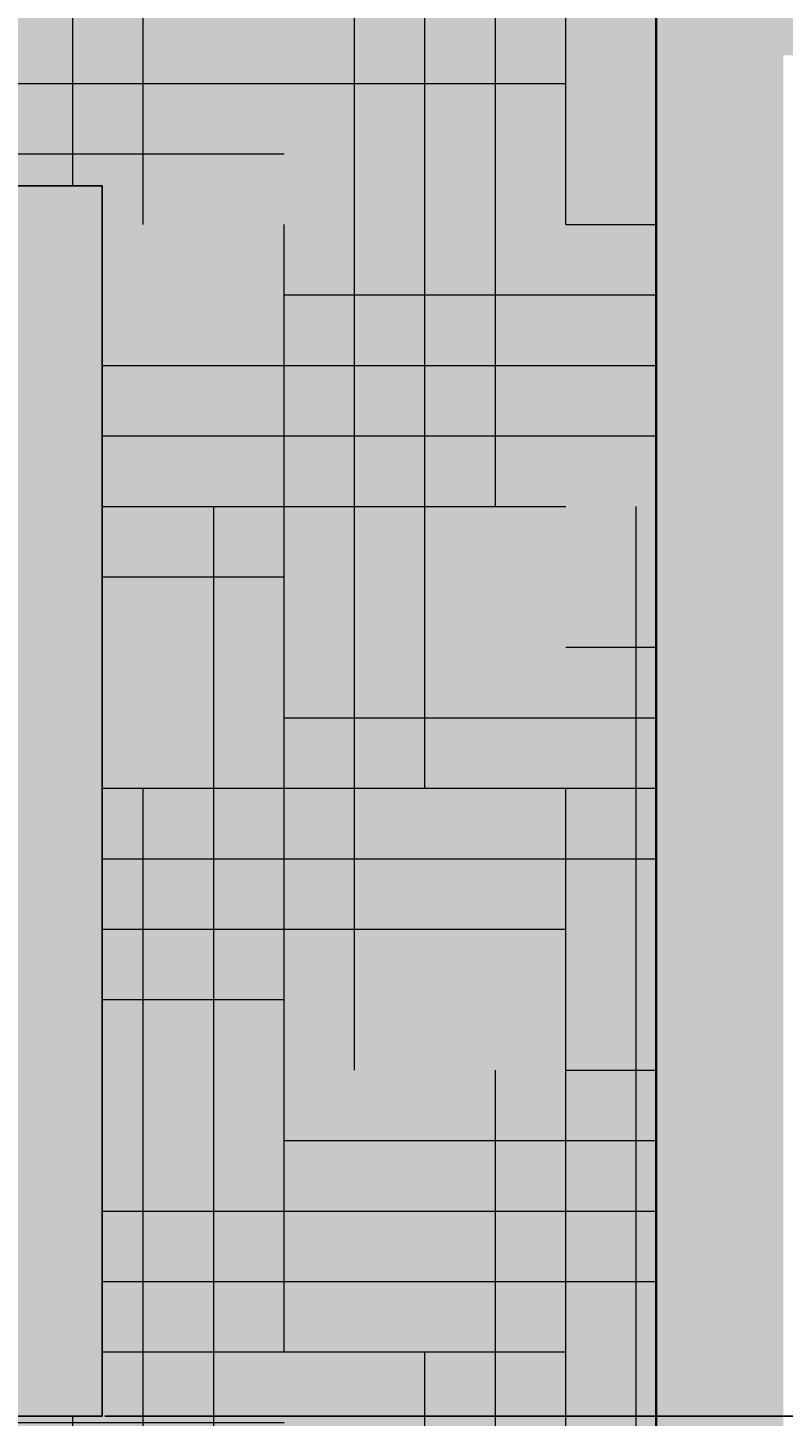
# Model space of a CAD drawing. Units: feet. Extents: x 2695 to 2912, y 795 to 1139.
# Tile 13 of 83: x 2756 to 2774, y 875 to 906. Entities that reach past the tile are written whole.
import ezdxf

# ---------------------------------------------------------------- set-up
doc = ezdxf.new("R2010")
doc.units = ezdxf.units.FT
for name, color, linetype, lineweight in [('A-ANNO-DIMS', 2, 'Continuous', 18), ('A-ELEV', 7, 'Continuous', 35), ('A-ELEV-PATT', 252, 'Continuous', 13), ('A-GLAZ', 4, 'Continuous', 25)]:
    doc.layers.add(name, color=color, linetype=linetype, lineweight=lineweight)
doc.styles.get("Standard").update_dxf_attribs({"font": 'arial.ttf'})
doc.dimstyles.get("Standard").update_dxf_attribs({"dimtxt": 0.18, "dimasz": 0.18, "dimexe": 0.18, "dimexo": 0.0625, "dimgap": 0.09, "dimtad": 0, "dimtih": 1, "dimtoh": 1, "dimdec": 1, "dimzin": 0, "dimdsep": 46, "dimlunit": 3, "dimtxsty": 'Standard', "dimcen": 0.09, "dimadec": 0, "dimazin": 0, "dimtfac": 1, "dimtdec": 1, "dimtofl": 0, "dimtmove": 0, "dimatfit": 3, "dimfxl": 1, "dimtolj": 1, "dimtzin": 0, "dimarcsym": 0})

# ---------------------------------------------------------------- blocks, each defined once
blk = doc.blocks.new('*D14')
at = {"layer": 'A-ANNO-DIMS', "color": 0, "lineweight": -2, "transparency": 16777216}
for p, q in [((2838.439, 905.514), (2911.424, 905.514)), ((2911.244, 905.334), (2911.244, 890.368)), ((2911.244, 875.037), (2911.244, 890.004)), ((2758.214, 874.857), (2911.424, 874.857))]:
    blk.add_line(p, q, dxfattribs=at)
at = {"layer": 'A-ANNO-DIMS', "color": 0, "transparency": 16777216}
for points in [[(2911.214, 905.334), (2911.274, 905.334), (2911.244, 905.514)], [(2911.214, 875.037), (2911.274, 875.037), (2911.244, 874.857)]]:
    blk.add_solid(points, dxfattribs=at)
at = {"layer": 'Defpoints', "color": 0, "transparency": 16777216}
for p in [(2838.377, 905.514), (2911.244, 905.514), (2758.151, 874.857)]:
    blk.add_point(p, dxfattribs=at)
at = {"layer": 'A-ANNO-DIMS', "color": 0, "transparency": 16777216, "insert": (2911.244, 890.186), "char_height": 0.18, "attachment_point": 5}
blk.add_mtext('\\A1;30.66', dxfattribs=at)
blk = doc.blocks.new('*D25')
at = {"layer": 'A-ANNO-DIMS', "color": 0, "lineweight": -2, "transparency": 16777216}
for p, q in [((2755.112, 936.868), (2755.112, 794.976)), ((2770.636, 936.868), (2770.636, 794.976)), ((2755.292, 795.156), (2762.419, 795.156)), ((2770.456, 795.156), (2763.329, 795.156))]:
    blk.add_line(p, q, dxfattribs=at)
at = {"layer": 'A-ANNO-DIMS', "color": 0, "transparency": 16777216}
for points in [[(2755.292, 795.186), (2755.292, 795.126), (2755.112, 795.156)], [(2770.456, 795.186), (2770.456, 795.126), (2770.636, 795.156)]]:
    blk.add_solid(points, dxfattribs=at)
at = {"layer": 'Defpoints', "color": 0, "transparency": 16777216}
for p in [(2755.112, 936.931), (2770.636, 936.931), (2770.636, 795.156)]:
    blk.add_point(p, dxfattribs=at)
at = {"layer": 'A-ANNO-DIMS', "color": 0, "transparency": 16777216, "insert": (2762.874, 795.156), "char_height": 0.18, "attachment_point": 5}
blk.add_mtext('\\A1;15.524', dxfattribs=at)

msp = doc.modelspace()

# ---------------------------------------------------------------- hatches: boundary and pattern name
at = {"layer": 'A-ELEV-PATT'}
h = msp.add_hatch(color=256, dxfattribs=at)
h.set_gradient(color1=(147, 149, 152), color2=(147, 149, 152), tint=1)
h.paths.add_polyline_path([(2770.6361, 1118.4096), (2710.6361, 1118.4096), (2710.6361, 1062.9306), (2770.6361, 1062.9306)])
h.paths.add_polyline_path([(2890.6361, 1103.3378), (2770.6361, 1103.3378), (2770.6361, 1062.9306), (2890.6361, 1062.9306)])
h.paths.add_polyline_path([(2730.7081, 1048.1052), (2755.1125, 1048.1052), (2755.1125, 936.9306), (2770.6361, 936.9306), (2770.6361, 1050.3105), (2715.8852, 1050.3105), (2715.8852, 936.9306), (2730.7081, 936.9306)])
h.paths.add_polyline_path([(2890.6361, 1050.3105), (2770.6361, 1050.3105), (2770.6361, 971.9673), (2778.0341, 971.9673), (2778.0341, 1020.8235), (2843.575, 1020.8235), (2843.575, 971.9673), (2890.6361, 971.9673)])
h.paths.add_polyline_path([(2888.1882, 970.7156), (2843.575, 970.7156), (2843.575, 964.8267), (2888.1882, 964.8267)])
h.paths.add_polyline_path([(2888.1882, 964.1328), (2843.575, 964.1328), (2843.575, 956.614), (2888.1882, 956.614)])
h.paths.add_polyline_path([(2888.1882, 955.9202), (2843.575, 955.9202), (2843.575, 949.2892), (2888.1882, 949.2892)])
h.paths.add_polyline_path([(2888.1882, 948.5954), (2843.575, 948.5954), (2843.575, 941.3507), (2888.1882, 941.3507)])
h.paths.add_polyline_path([(2888.1882, 940.6569), (2843.575, 940.6569), (2843.575, 936.9306), (2888.1882, 936.9306)])
h.paths.add_polyline_path([(2890.6361, 970.7156), (2888.9368, 970.7156), (2888.9368, 964.8267), (2890.6361, 964.8267)])
h.paths.add_polyline_path([(2890.6361, 964.1328), (2888.9368, 964.1328), (2888.9368, 956.614), (2890.6361, 956.614)])
h.paths.add_polyline_path([(2890.6361, 955.9202), (2888.9368, 955.9202), (2888.9368, 949.2892), (2890.6361, 949.2892)])
h.paths.add_polyline_path([(2890.6361, 940.6569), (2888.9368, 940.6569), (2888.9368, 936.9306), (2890.6361, 936.9306)])
h.paths.add_polyline_path([(2890.6361, 948.5954), (2888.9368, 948.5954), (2888.9368, 941.3507), (2890.6361, 941.3507)])
h.paths.add_polyline_path([(2772.5216, 970.7156), (2770.6361, 970.7156), (2770.6361, 964.8267), (2772.5216, 964.8267)])
h.paths.add_polyline_path([(2772.5216, 964.1328), (2770.6361, 964.1328), (2770.6361, 956.614), (2772.5216, 956.614)])
h.paths.add_polyline_path([(2772.5216, 955.9202), (2770.6361, 955.9202), (2770.6361, 949.2892), (2772.5216, 949.2892)])
h.paths.add_polyline_path([(2772.5216, 948.5954), (2770.6361, 948.5954), (2770.6361, 941.3507), (2772.5216, 941.3507)])
h.paths.add_polyline_path([(2772.5216, 940.6569), (2770.6361, 940.6569), (2770.6361, 936.9306), (2772.5216, 936.9306)])
h.paths.add_polyline_path([(2778.0341, 940.6569), (2773.2702, 940.6569), (2773.2702, 936.9306), (2778.0341, 936.9306)])
h.paths.add_polyline_path([(2778.0341, 970.7156), (2773.2702, 970.7156), (2773.2702, 964.8267), (2778.0341, 964.8267)])
h.paths.add_polyline_path([(2778.0341, 964.1328), (2773.2702, 964.1328), (2773.2702, 956.614), (2778.0341, 956.614)])
h.paths.add_polyline_path([(2778.0341, 955.9202), (2773.2702, 955.9202), (2773.2702, 949.2892), (2778.0341, 949.2892)])
h.paths.add_polyline_path([(2778.0341, 948.5954), (2773.2702, 948.5954), (2773.2702, 941.3507), (2778.0341, 941.3507)])
h.paths.add_polyline_path([(2810.0407, 940.6569), (2780.0341, 940.6569), (2780.0341, 936.9306), (2810.0407, 936.9306)])
h.paths.add_polyline_path([(2890.6361, 924.3105), (2770.6361, 924.3105), (2770.6361, 810.9306), (2773.5029, 810.9306), (2773.5029, 905.5143), (2805.9398, 905.5143), (2838.3767, 905.5143), (2838.3767, 810.9306), (2890.6361, 810.9306)])
h = msp.add_hatch(color=256, dxfattribs=at)
h.set_gradient(color2=(0, 0, 0), tint=1)
h.paths.add_polyline_path([(2772.5216, 971.9673), (2770.6361, 971.9673), (2770.6361, 970.7156), (2772.5216, 970.7156)])
h.paths.add_polyline_path([(2773.2702, 971.9673), (2772.5216, 971.9673), (2772.5216, 970.7156), (2773.2702, 970.7156)])
h.paths.add_polyline_path([(2778.0341, 971.9673), (2773.2702, 971.9673), (2773.2702, 970.7156), (2778.0341, 970.7156)])
h.paths.add_polyline_path([(2780.0341, 971.9673), (2778.0341, 971.9673), (2778.0341, 970.7156), (2780.0341, 970.7156)])
h.paths.add_polyline_path([(2841.575, 971.9673), (2780.0341, 971.9673), (2780.0341, 970.7156), (2841.575, 970.7156)])
h.paths.add_polyline_path([(2843.575, 971.9673), (2841.575, 971.9673), (2841.575, 970.7156), (2843.575, 970.7156)])
h.paths.add_polyline_path([(2888.1882, 971.9673), (2843.575, 971.9673), (2843.575, 970.7156), (2888.1882, 970.7156)])
h.paths.add_polyline_path([(2888.9368, 971.9673), (2888.1882, 971.9673), (2888.1882, 970.7156), (2888.9368, 970.7156)], flags=17)
h.paths.add_polyline_path([(2890.6361, 971.9673), (2888.9368, 971.9673), (2888.9368, 970.7156), (2890.6361, 970.7156)])
h.paths.add_polyline_path([(2888.9368, 971.9673), (2888.1882, 971.9673), (2888.1882, 964.8267), (2888.9368, 964.8267)])
h.paths.add_polyline_path([(2888.9368, 964.8267), (2888.1882, 964.8267), (2888.1882, 964.1328), (2888.9368, 964.1328)])
h.paths.add_polyline_path([(2890.6361, 964.8267), (2888.9368, 964.8267), (2888.9368, 964.1328), (2890.6361, 964.1328)])
h.paths.add_polyline_path([(2888.1882, 964.8267), (2770.6361, 964.8267), (2770.6361, 964.1328), (2888.1882, 964.1328)])
h.paths.add_polyline_path([(2888.9368, 964.1328), (2888.1882, 964.1328), (2888.1882, 936.9306), (2888.9368, 936.9306)])
h.paths.add_polyline_path([(2890.6361, 956.614), (2888.9368, 956.614), (2888.9368, 955.9202), (2890.6361, 955.9202)])
h.paths.add_polyline_path([(2888.1882, 956.614), (2770.6361, 956.614), (2770.6361, 955.9202), (2888.1882, 955.9202)])
h.paths.add_polyline_path([(2890.6361, 949.2892), (2888.9368, 949.2892), (2888.9368, 948.5954), (2890.6361, 948.5954)])
h.paths.add_polyline_path([(2888.1882, 949.2892), (2770.6361, 949.2892), (2770.6361, 948.5954), (2888.1882, 948.5954)])
h.paths.add_polyline_path([(2890.6361, 941.3507), (2888.9368, 941.3507), (2888.9368, 940.6569), (2890.6361, 940.6569)])
h.paths.add_polyline_path([(2888.1882, 941.3507), (2770.6361, 941.3507), (2770.6361, 940.6569), (2888.1882, 940.6569)])
h.paths.add_polyline_path([(2773.2702, 970.7156), (2772.5216, 970.7156), (2772.5216, 964.8267), (2773.2702, 964.8267)])
h.paths.add_polyline_path([(2773.2702, 964.1328), (2772.5216, 964.1328), (2772.5216, 956.614), (2773.2702, 956.614)])
h.paths.add_polyline_path([(2773.2702, 955.9202), (2772.5216, 955.9202), (2772.5216, 936.9306), (2773.2702, 936.9306)])
h.paths.add_polyline_path([(2810.7893, 970.7156), (2810.0407, 970.7156), (2810.0407, 964.8267), (2810.7893, 964.8267)], flags=17)
h.paths.add_polyline_path([(2810.7893, 964.1328), (2810.0407, 964.1328), (2810.0407, 956.614), (2810.7893, 956.614)], flags=17)
h.paths.add_polyline_path([(2810.7893, 955.9202), (2810.0407, 955.9202), (2810.0407, 949.2892), (2810.7893, 949.2892)], flags=17)
h.paths.add_polyline_path([(2810.7893, 971.9673), (2810.0407, 971.9673), (2810.0407, 941.3507), (2810.7893, 941.3507)])
h.paths.add_polyline_path([(2810.7893, 940.6569), (2810.0407, 940.6569), (2810.0407, 936.9306), (2810.7893, 936.9306)])
h.paths.add_polyline_path([(2780.0341, 1018.8235), (2841.575, 1018.8235), (2841.575, 971.9673), (2843.575, 971.9673), (2843.575, 1020.8235), (2778.0341, 1020.8235), (2778.0341, 971.9673), (2780.0341, 971.9673)])
h.paths.add_polyline_path([(2780.0341, 970.7156), (2778.0341, 970.7156), (2778.0341, 964.8267), (2780.0341, 964.8267)])
h.paths.add_polyline_path([(2780.0341, 964.1328), (2778.0341, 964.1328), (2778.0341, 956.614), (2780.0341, 956.614)])
h.paths.add_polyline_path([(2780.0341, 955.9202), (2778.0341, 955.9202), (2778.0341, 949.2892), (2780.0341, 949.2892)])
h.paths.add_polyline_path([(2780.0341, 948.5954), (2778.0341, 948.5954), (2778.0341, 941.3507), (2780.0341, 941.3507)])
h.paths.add_polyline_path([(2780.0341, 940.6569), (2778.0341, 940.6569), (2778.0341, 936.9306), (2780.0341, 936.9306)])
h.paths.add_polyline_path([(2843.575, 940.6569), (2841.575, 940.6569), (2841.575, 936.9306), (2843.575, 936.9306)])
h.paths.add_polyline_path([(2843.575, 948.5954), (2841.575, 948.5954), (2841.575, 941.3507), (2843.575, 941.3507)])
h.paths.add_polyline_path([(2843.575, 970.7156), (2841.575, 970.7156), (2841.575, 964.8267), (2843.575, 964.8267)])
h.paths.add_polyline_path([(2843.575, 964.1328), (2841.575, 964.1328), (2841.575, 956.614), (2843.575, 956.614)])
h.paths.add_polyline_path([(2843.575, 955.9202), (2841.575, 955.9202), (2841.575, 949.2892), (2843.575, 949.2892)])
h.paths.add_polyline_path([(2805.0538, 874.1057), (2803.9681, 874.1057), (2803.9681, 846.2857), (2805.0538, 846.2857)])
h.paths.add_polyline_path([(2758.1515, 902.577), (2724.1893, 902.577), (2724.1893, 874.8571), (2758.1515, 874.8571)])
h.paths.add_polyline_path([(2726.1893, 900.577), (2756.1515, 900.577), (2756.1515, 876.8571), (2726.1893, 876.8571)], flags=16)
h.paths.add_polyline_path([(2740.7302, 900.577), (2741.6105, 900.577), (2741.6105, 876.8571), (2740.7302, 876.8571)], flags=0)
h = msp.add_hatch(color=256, dxfattribs=at)
h.set_gradient(color1=(255, 255, 255))
h.paths.add_polyline_path([(2770.6361, 924.3105), (2716.5358, 924.3105), (2716.5358, 810.9306), (2770.6361, 810.9306)])
h.paths.add_polyline_path([(2758.1515, 902.577), (2758.1515, 874.8571), (2724.1893, 874.8571), (2724.1893, 902.577)], flags=16)
h.paths.add_polyline_path([(2756.1515, 900.577), (2756.1515, 876.8571), (2726.1893, 876.8571), (2726.1893, 900.577)], flags=0)
h.paths.add_polyline_path([(2740.7302, 900.577), (2741.6105, 900.577), (2741.6105, 876.8571), (2740.7302, 876.8571)], flags=0)
h = msp.add_hatch(dxfattribs=at)
h.set_pattern_fill('HOUND', color=256, style=0)
h.paths.add_polyline_path([(2770.6361, 924.3105), (2716.5358, 924.3105), (2716.5358, 810.9306), (2770.6361, 810.9306)])
h.paths.add_polyline_path([(2724.1893, 874.8571), (2724.1893, 902.577), (2758.1515, 902.577), (2758.1515, 874.8571)], flags=16)
h.paths.add_polyline_path([(2756.1515, 876.8571), (2726.1893, 876.8571), (2726.1893, 900.577), (2756.1515, 900.577)], flags=0)
h.paths.add_polyline_path([(2741.6105, 876.8571), (2740.7302, 876.8571), (2740.7302, 900.577), (2741.6105, 900.577)], flags=0)

# ---------------------------------------------------------------- linework, layer by layer
at = {"layer": 'A-ELEV'}
for p, q in [((2770.6361, 924.3105), (2770.6361, 810.9306)), ((2770.6361, 810.9306), (2770.6361, 924.3105))]:
    msp.add_line(p, q, dxfattribs=at)
msp.add_lwpolyline([(2716.5358, 924.3105), (2770.6361, 924.3105), (2770.6361, 810.9306), (2716.5358, 810.9306)], close=True, dxfattribs=at)
at = {"layer": 'A-GLAZ'}
for p, q in [((2724.1893, 902.577), (2758.1515, 902.577)), ((2758.1515, 902.577), (2758.1515, 874.8571)), ((2758.1515, 874.8571), (2724.1893, 874.8571))]:
    msp.add_line(p, q, dxfattribs=at)
msp.add_lwpolyline([(2724.1893, 902.577), (2758.1515, 902.577), (2758.1515, 874.8571), (2724.1893, 874.8571)], close=True, dxfattribs=at)

# ---------------------------------------------------------------- dimensions: what is measured, and where the dimension line sits
at = {"layer": 'A-ANNO-DIMS'}
dim = msp.add_linear_dim(base=(2770.6361, 795.1556), p1=(2755.1125, 936.9306), p2=(2770.6361, 936.9306), dimstyle='Standard', override={"dimdec": 3, "dimlfac": 1, "dimrnd": 0, "dimzin": 0, "dimdsep": 46, "dimlunit": 2}, dxfattribs=at)
dim.commit()
dim.dimension.update_dxf_attribs({"geometry": '*D25', "text_midpoint": (2762.8743, 795.1556)})
dim = msp.add_linear_dim(base=(2911.2444, 905.5143), p1=(2758.1515, 874.8571), p2=(2838.3767, 905.5143), angle=90, dimstyle='Standard', override={"dimdec": 2, "dimlfac": 1, "dimrnd": 0, "dimzin": 0, "dimdsep": 46, "dimlunit": 2}, dxfattribs=at)
dim.commit()
dim.dimension.update_dxf_attribs({"geometry": '*D14', "text_midpoint": (2911.2444, 890.1857)})

doc.saveas('drawing.dxf')
